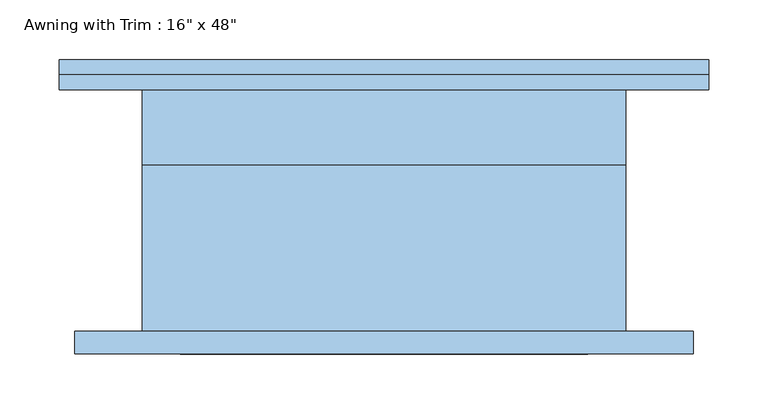
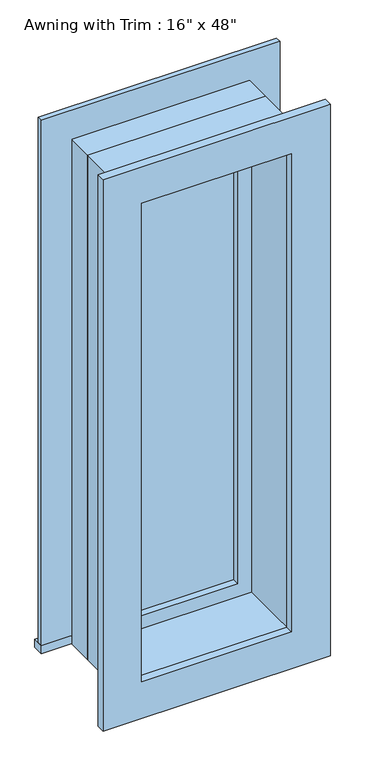
"""IFC4 building model written with IfcOpenShell, lengths in millimetres: window geometry."""

from ifc_helpers import new_model, si_unit, frame, origin, place, context, project, spatial, polyline, outline, extrude, source, transform, mapped, element, save


def window_a765b88f(model_context):
    return source(origin(), model_context, "Body", "SweptSolid", [
        extrude(outline(polyline([(-273.05, 127.0), (273.05, 127.0), (273.05, 101.6), (-273.05, 101.6), (-273.05, 127.0)])), frame((0.0, 0.0, 914.4), z_axis=(0.0, 0.0, 1.0), x_axis=(1.0, 0.0, 0.0)), (0.0, 0.0, 1.0), 19.05),
        extrude(outline(polyline([(2114.55, -184.15), (2114.55, 184.15), (933.45, 184.15), (933.45, 273.05), (2203.45, 273.05), (2203.45, -273.05), (933.45, -273.05), (933.45, -184.15), (2114.55, -184.15)])), frame((0.0, 101.6, 0.0), z_axis=(0.0, 1.0, 0.0), x_axis=(0.0, 0.0, 1.0)), (0.0, 0.0, 1.0), 12.7),
        extrude(outline(polyline([(2190.75, 260.35), (2190.75, -260.35), (857.25, -260.35), (857.25, 260.35), (2190.75, 260.35)]), holes=[polyline([(2101.85, 171.45), (946.15, 171.45), (946.15, -171.45), (2101.85, -171.45), (2101.85, 171.45)])]), frame((0.0, -120.65, 0.0), z_axis=(0.0, 1.0, 0.0), x_axis=(0.0, 0.0, 1.0)), (0.0, 0.0, 1.0), 19.05),
        extrude(outline(polyline([(139.7, 53.975), (-139.7, 53.975), (-139.7, 66.675), (139.7, 66.675), (139.7, 53.975)])), frame((0.0, 0.0, 977.9), z_axis=(0.0, 0.0, 1.0), x_axis=(1.0, 0.0, 0.0)), (0.0, 0.0, 1.0), 1092.2),
        extrude(outline(polyline([(2114.55, -184.15), (933.45, -184.15), (933.45, 184.15), (2114.55, 184.15), (2114.55, -184.15)]), holes=[polyline([(2070.1, -139.7), (2070.1, 139.7), (977.9, 139.7), (977.9, -139.7), (2070.1, -139.7)])]), frame((0.0, 38.1, 0.0), z_axis=(0.0, 1.0, 0.0), x_axis=(0.0, 0.0, 1.0)), (0.0, 0.0, 1.0), 44.45),
        extrude(outline(polyline([(2133.6, -203.2), (914.4, -203.2), (914.4, 203.2), (2133.6, 203.2), (2133.6, -203.2)]), holes=[polyline([(2101.85, -171.45), (2101.85, 171.45), (946.15, 171.45), (946.15, -171.45), (2101.85, -171.45)])]), frame((0.0, -101.6, 0.0), z_axis=(0.0, 1.0, 0.0), x_axis=(0.0, 0.0, 1.0)), (0.0, 0.0, 1.0), 139.7),
        extrude(outline(polyline([(2133.6, 203.2), (2133.6, -203.2), (914.4, -203.2), (914.4, 203.2), (2133.6, 203.2)]), holes=[polyline([(2114.55, 184.15), (933.45, 184.15), (933.45, -184.15), (2114.55, -184.15), (2114.55, 184.15)])]), frame((0.0, 38.1, 0.0), z_axis=(0.0, 1.0, 0.0), x_axis=(0.0, 0.0, 1.0)), (0.0, 0.0, 1.0), 63.5),
    ])


if __name__ == "__main__":
    model = new_model("IFC4")
    model_context = context("Model", 3, world=origin())
    ifc_project = project(units=[si_unit("LENGTHUNIT", "METRE", prefix="MILLI")], contexts=[model_context])
    site = spatial("IfcSite", under=ifc_project)
    building = spatial("IfcBuilding", under=site)
    placement = place(None, origin())
    window_shape = window_a765b88f(model_context)
    element("IfcWindow", 1, ObjectType="Awning with Trim : 16\" x 48\"", at=placement, inside=building, context=model_context, shape_type="MappedRepresentation", body=[
        mapped(window_shape, transform((0.0, 0.0, 0.0), x_axis=(1.0, 0.0, 0.0), y_axis=(0.0, 1.0, 0.0), z_axis=(0.0, 0.0, 1.0))),
    ])
    save(model, "model.ifc")

# Revit data of these elements
# Type "Awning with Trim : 16\" x 48\""
#   Type Mark = "14"
#   Construction Type Id = "GSP4R"
#   Assembly Code = "B2020100"
#   Analytic Construction = "1/8 in Pilkington single glazing"
#   Visual Light Transmittance = 0.9
#   Solar Heat Gain Coefficient = 0.78
#   Heat Transfer Coefficient (U) = 0.6496 BTU/(h·ft²·°F)
#   Height = 4' - 0"
#   Default Sill Height = 3' - 0"
#   Trim Projection - Ext. = 0' - 0 1/2"
#   Trim Projection - Int. = 0' - 0 3/4"
#   Trim Width - Exterior = 0' - 3 1/2"
#   Trim Width - Interior = 0' - 3 1/2"
#   Width = 1' - 4"
#   Window Inset = 0' - 0 3/4"
#   Define Thermal Properties by = 1
#   Glass Pane Material = Glass
#   Sash Material = Sash
#   Trim Exterior Material = Trim
#   Trim Interior Material = Trim
#   Wall Closure = (empty or 0)
# Element 1 (IfcWindow, "Awning with Trim : 16\" x 48\"")
#   Materials on its faces: "Sash", "Trim", "Glass"
# Materials
#   "Glass": class "Glass", colour RGB 0 128 192, transparency 0.75, Description = "Soda Lime Glass", Cost = 0
#   "Sash": class "Wood", colour RGB 224 178 126, transparency 0
#   "Trim": class "Wood", colour RGB 224 178 126, transparency 0
